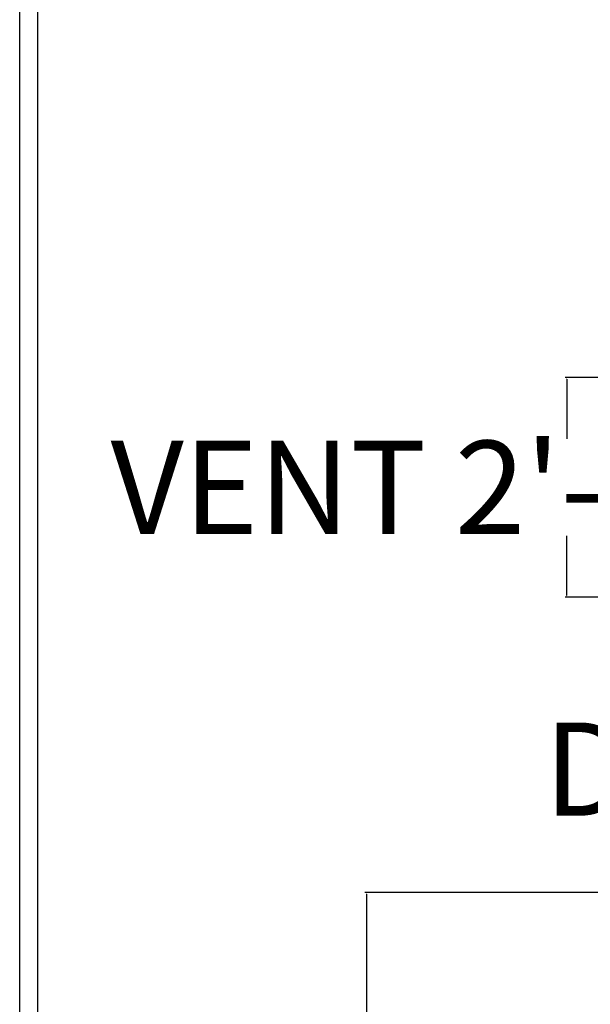
# Model space of a CAD drawing. Units: inches. Extents: x 1812 to 2791, y 2306 to 2959.
# Tile 6 of 8: x 2391 to 2453, y 2748 to 2856. Entities that reach past the tile are written whole.
import ezdxf

# ---------------------------------------------------------------- set-up
doc = ezdxf.new("R2010")
doc.units = ezdxf.units.IN
doc.layers.get('Defpoints').update_dxf_attribs({"lineweight": 50})
doc.layers.add('A-ANNO-DIMS', color=2, linetype='Continuous', lineweight=18)
doc.layers.add('A-ANNO-TTLB', color=7, linetype='Continuous', lineweight=25)
doc.styles.get("Standard").update_dxf_attribs({"font": 'arial.ttf'})
doc.dimstyles.get("Standard").update_dxf_attribs({"dimtxt": 10.18, "dimasz": 0.18, "dimexe": 0.18, "dimexo": 0.0625, "dimgap": 0.09, "dimtad": 0, "dimtih": 1, "dimtoh": 1, "dimdec": 0, "dimzin": 0, "dimdsep": 46, "dimlunit": 3, "dimtxsty": 'Standard', "dimcen": 0.09, "dimadec": 0, "dimazin": 0, "dimtfac": 1, "dimtdec": 0, "dimtofl": 0, "dimtmove": 0, "dimatfit": 3, "dimfxl": 1, "dimtolj": 1, "dimtzin": 0, "dimarcsym": 0})

# ---------------------------------------------------------------- blocks, each defined once
blk = doc.blocks.new('SHEET-FRAME-RESIDENCE')
blk.add_lwpolyline([(0.000131823559741, 632.8005012919775), (378.7609620870107, 632.8005012919775), (378.7609620870107, 0.0003856501880364), (0.000131823559741, 0.0003856501880364)], close=True)
blk.add_lwpolyline([(2.00013182355974, 71.32450104412055), (2.00013182355974, 630.8005012919775), (376.7609620870107, 630.8005012919775), (376.7609620870107, 71.32450104412055)])
blk = doc.blocks.new('*D48')
at = {"layer": 'A-ANNO-DIMS', "color": 0, "lineweight": -2, "transparency": 16777216}
for p, q in [((2454.200753859796, 2816.957881357629), (2450.483253859797, 2816.957881357629)), ((2450.663253859797, 2816.777881357629), (2450.663253859797, 2810.245514372636)), ((2450.663253859797, 2793.137881357629), (2450.663253859797, 2799.670248342622)), ((2454.200753859796, 2792.957881357629), (2450.483253859797, 2792.957881357629))]:
    blk.add_line(p, q, dxfattribs=at)
at = {"layer": 'A-ANNO-DIMS', "color": 0, "transparency": 16777216}
for points in [[(2450.633253859797, 2816.777881357629), (2450.693253859797, 2816.777881357629), (2450.663253859797, 2816.957881357629)], [(2450.633253859797, 2793.137881357629), (2450.693253859797, 2793.137881357629), (2450.663253859797, 2792.957881357629)]]:
    blk.add_solid(points, dxfattribs=at)
at = {"layer": 'Defpoints', "color": 0, "transparency": 16777216}
for p in [(2450.663253859797, 2816.957881357629), (2454.263253859796, 2816.957881357629), (2454.263253859796, 2792.957881357629)]:
    blk.add_point(p, dxfattribs=at)
at = {"layer": 'A-ANNO-DIMS', "color": 0, "transparency": 16777216, "insert": (2450.663253859797, 2804.957881357628), "char_height": 10.18, "attachment_point": 5}
blk.add_mtext('\\A1;VENT 2\'-0" TYP.', dxfattribs=at)
blk = doc.blocks.new('*D60')
at = {"layer": 'A-ANNO-DIMS', "color": 0, "lineweight": -2, "transparency": 16777216}
for p, q in [((2505.177694196558, 2790.74953182163), (2500.089565400664, 2790.74953182163)), ((2500.269565400663, 2790.56953182163), (2500.269565400663, 2779.537842838497)), ((2500.269565400663, 2757.792006515665), (2500.269565400663, 2768.823695498797)), ((2505.177694196558, 2757.612006515665), (2500.089565400664, 2757.612006515665))]:
    blk.add_line(p, q, dxfattribs=at)
at = {"layer": 'A-ANNO-DIMS', "color": 0, "transparency": 16777216}
for points in [[(2500.239565400664, 2790.56953182163), (2500.299565400664, 2790.56953182163), (2500.269565400663, 2790.74953182163)], [(2500.239565400664, 2757.792006515665), (2500.299565400664, 2757.792006515665), (2500.269565400663, 2757.612006515665)]]:
    blk.add_solid(points, dxfattribs=at)
at = {"layer": 'Defpoints', "color": 0, "transparency": 16777216}
for p in [(2500.269565400663, 2790.74953182163), (2505.240194196558, 2790.74953182163), (2505.240194196558, 2757.612006515665)]:
    blk.add_point(p, dxfattribs=at)
at = {"layer": 'A-ANNO-DIMS', "color": 0, "transparency": 16777216, "insert": (2500.269565400663, 2774.180769168646), "char_height": 10.18, "attachment_point": 5}
blk.add_mtext('\\A1;DOOR 2\'-9" TYP.', dxfattribs=at)
blk = doc.blocks.new('*D73')
at = {"layer": 'A-ANNO-DIMS', "color": 0, "lineweight": -2, "transparency": 16777216}
for p, q in [((2454.218562000001, 2760.694666000001), (2428.586486000002, 2760.694666000001)), ((2428.766486000002, 2760.514666000001), (2428.766486000002, 2692.848797196454)), ((2428.766486000002, 2614.781264000001), (2428.766486000002, 2682.447132803548)), ((2454.176191000001, 2614.601264000001), (2428.586486000002, 2614.601264000001))]:
    blk.add_line(p, q, dxfattribs=at)
at = {"layer": 'A-ANNO-DIMS', "color": 0, "transparency": 16777216}
for points in [[(2428.736486000002, 2760.514666000001), (2428.796486000002, 2760.514666000001), (2428.766486000002, 2760.694666000001)], [(2428.736486000002, 2614.781264000001), (2428.796486000002, 2614.781264000001), (2428.766486000002, 2614.601264000001)]]:
    blk.add_solid(points, dxfattribs=at)
at = {"layer": 'Defpoints', "color": 0, "transparency": 16777216}
for p in [(2428.766486000002, 2760.694666000001), (2454.281062000001, 2760.694666000001), (2454.238691000001, 2614.601264000001)]:
    blk.add_point(p, dxfattribs=at)
at = {"layer": 'A-ANNO-DIMS', "color": 0, "transparency": 16777216, "insert": (2428.766486000002, 2687.647965), "char_height": 10.18, "attachment_point": 5}
blk.add_mtext('\\A1;12\'-2"', dxfattribs=at)

msp = doc.modelspace()

# ---------------------------------------------------------------- block references
at = {"layer": 'A-ANNO-TTLB'}
msp.add_blockref('SHEET-FRAME-RESIDENCE', (2390.832750765552, 2326.134678289167), dxfattribs=at)

# ---------------------------------------------------------------- dimensions: what is measured, and where the dimension line sits
at = {"layer": 'A-ANNO-DIMS'}
for base, p1, p2, text, picture, middle in [((2450.663253859797, 2816.957881357629), (2454.263253859795, 2792.957881357628), (2454.263253859795, 2816.957881357629), 'VENT <> TYP.', '*D48', (2450.663253859797, 2804.957881357628)), ((2500.269565400663, 2790.74953182163), (2505.240194196556, 2757.612006515664), (2505.240194196556, 2790.749531821629), 'DOOR <> TYP.', '*D60', (2500.269565400663, 2774.180769168646))]:
    dim = msp.add_linear_dim(base=base, p1=p1, p2=p2, angle=90, text=text, dimstyle='Standard', override={"dimdec": 1, "dimlfac": 1, "dimrnd": 0, "dimzin": 1, "dimdsep": 46, "dimlunit": 4, "dimfrac": 2}, dxfattribs=at)
    dim.commit()
    dim.dimension.update_dxf_attribs({"geometry": picture, "text_midpoint": middle})
dim = msp.add_linear_dim(base=(2428.766486000002, 2760.694666000001), p1=(2454.238691, 2614.601264), p2=(2454.281062, 2760.694666), angle=90, dimstyle='Standard', override={"dimdec": 1, "dimlfac": 1, "dimrnd": 0, "dimzin": 1, "dimdsep": 46, "dimlunit": 4, "dimfrac": 2}, dxfattribs=at)
dim.commit()
dim.dimension.update_dxf_attribs({"geometry": '*D73', "text_midpoint": (2428.766486000002, 2687.647965)})

doc.saveas('drawing.dxf')
